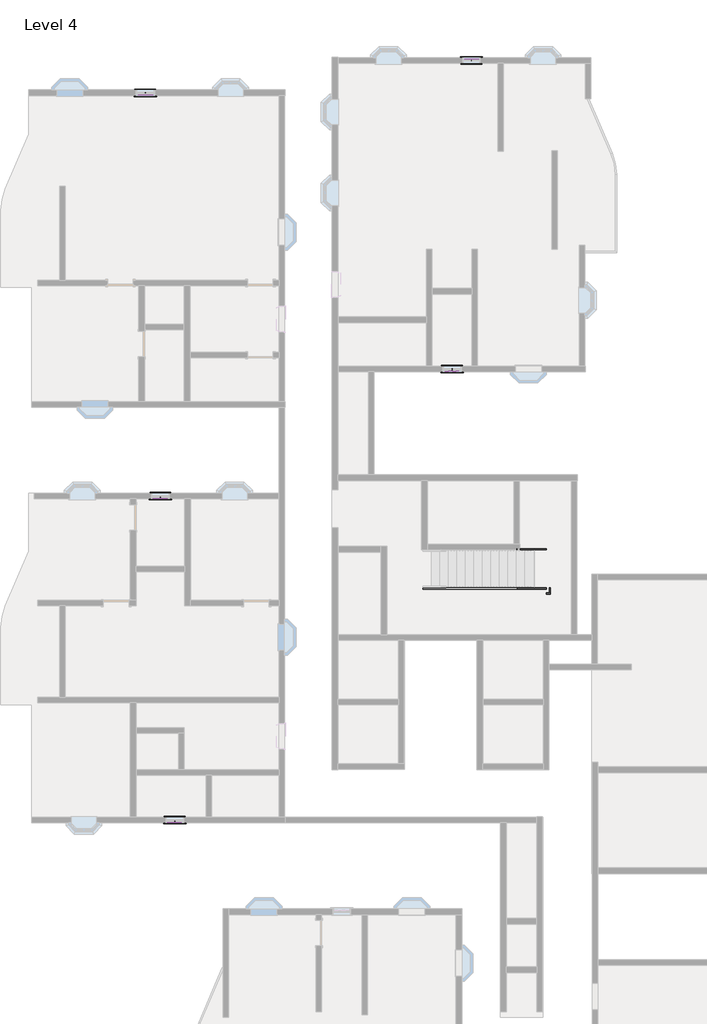
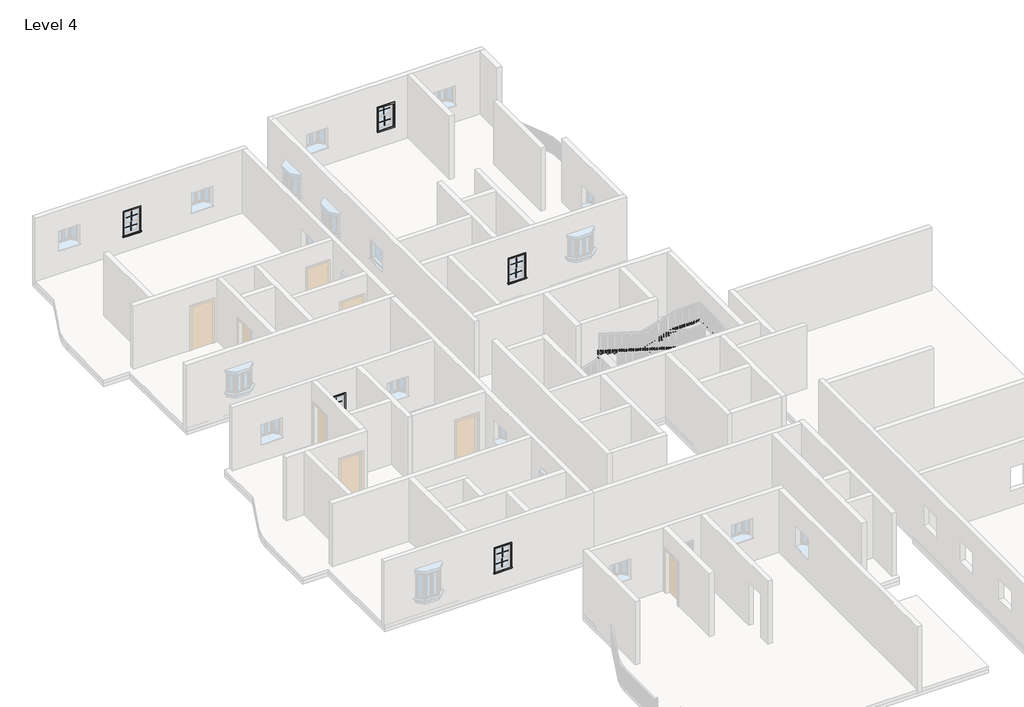
# One storey, part 14 of 14: 20 proxies, 6 members.
"""IFC4 building model written with IfcOpenShell, lengths in millimetres."""

from ifc_helpers import new_model, si_unit, frame, origin, place, context, project, spatial, polyline, outline, extrude, transform, mapped, element, save
from components import muntin_pattern_2x2_muntin_pattern_2x2_c35c595f, trim_window_exterior_flat_with_sill_e38017c9, trim_window_interior_flat_picture_frame_d728ed12

model = new_model("IFC4")

# Units and contexts
model_context = context("Model", 3, world=origin())
ifc_project = project(units=[si_unit("LENGTHUNIT", "METRE", prefix="MILLI")], contexts=[model_context])

# Site, building, storey
site = spatial("IfcSite", under=ifc_project)
building = spatial("IfcBuilding", under=site)
storey = spatial("IfcBuildingStorey", under=building, Name="Level 4", Elevation=9144.0)

# Proxies
placement = place(None, origin())
muntin_pattern_2x2_muntin_pattern_2x2_shape = muntin_pattern_2x2_muntin_pattern_2x2_c35c595f(model_context)
element("IfcBuildingElementProxy", 1, Name="Muntin Pattern_2x2 : Muntin Pattern_2x2", ObjectType="Muntin Pattern_2x2 : Muntin Pattern_2x2", at=placement, inside=storey, context=model_context, shape_type="MappedRepresentation", body=[
    mapped(muntin_pattern_2x2_muntin_pattern_2x2_shape, transform((-14639.3891351, 14368.0833494, 10614.025), x_axis=(-1.0, 0.0, 0.0), y_axis=(0.0, -1.0, 0.0), z_axis=(0.0, 0.0, 1.0))),
])
element("IfcBuildingElementProxy", 2, Name="Muntin Pattern_2x2 : Muntin Pattern_2x2", ObjectType="Muntin Pattern_2x2 : Muntin Pattern_2x2", at=placement, inside=storey, context=model_context, shape_type="MappedRepresentation", body=[
    mapped(muntin_pattern_2x2_muntin_pattern_2x2_shape, transform((-14639.3891351, 14412.5333494, 10134.6), x_axis=(-1.0, 0.0, 0.0), y_axis=(0.0, -1.0, 0.0), z_axis=(0.0, 0.0, 1.0))),
])
element("IfcBuildingElementProxy", 3, Name="Muntin Pattern_2x2 : Muntin Pattern_2x2", ObjectType="Muntin Pattern_2x2 : Muntin Pattern_2x2", at=placement, inside=storey, context=model_context, shape_type="MappedRepresentation", body=[
    mapped(muntin_pattern_2x2_muntin_pattern_2x2_shape, transform((-14125.0391351, 2785.6833494, 10614.025), x_axis=(-1.0, 0.0, 0.0), y_axis=(0.0, -1.0, 0.0), z_axis=(0.0, 0.0, 1.0))),
])
element("IfcBuildingElementProxy", 4, Name="Muntin Pattern_2x2 : Muntin Pattern_2x2", ObjectType="Muntin Pattern_2x2 : Muntin Pattern_2x2", at=placement, inside=storey, context=model_context, shape_type="MappedRepresentation", body=[
    mapped(muntin_pattern_2x2_muntin_pattern_2x2_shape, transform((-14125.0391351, 2830.1333494, 10134.6), x_axis=(-1.0, 0.0, 0.0), y_axis=(0.0, -1.0, 0.0), z_axis=(0.0, 0.0, 1.0))),
])
element("IfcBuildingElementProxy", 5, Name="Muntin Pattern_2x2 : Muntin Pattern_2x2", ObjectType="Muntin Pattern_2x2 : Muntin Pattern_2x2", at=placement, inside=storey, context=model_context, shape_type="MappedRepresentation", body=[
    mapped(muntin_pattern_2x2_muntin_pattern_2x2_shape, transform((-4206.3391351, 18910.0465905, 10614.025), x_axis=(-1.0, 0.0, 0.0), y_axis=(0.0, -1.0, 0.0), z_axis=(0.0, 0.0, 1.0))),
])
element("IfcBuildingElementProxy", 6, Name="Muntin Pattern_2x2 : Muntin Pattern_2x2", ObjectType="Muntin Pattern_2x2 : Muntin Pattern_2x2", at=placement, inside=storey, context=model_context, shape_type="MappedRepresentation", body=[
    mapped(muntin_pattern_2x2_muntin_pattern_2x2_shape, transform((-4206.3391351, 18954.4965905, 10134.6), x_axis=(-1.0, 0.0, 0.0), y_axis=(0.0, -1.0, 0.0), z_axis=(0.0, 0.0, 1.0))),
])
element("IfcBuildingElementProxy", 7, Name="Muntin Pattern_2x2 : Muntin Pattern_2x2", ObjectType="Muntin Pattern_2x2 : Muntin Pattern_2x2", at=placement, inside=storey, context=model_context, shape_type="MappedRepresentation", body=[
    mapped(muntin_pattern_2x2_muntin_pattern_2x2_shape, transform((-3514.1891351, 30066.9965905, 10614.025), x_axis=(1.0, 0.0, 0.0), y_axis=(0.0, 1.0, 0.0), z_axis=(0.0, 0.0, 1.0))),
])
element("IfcBuildingElementProxy", 8, Name="Muntin Pattern_2x2 : Muntin Pattern_2x2", ObjectType="Muntin Pattern_2x2 : Muntin Pattern_2x2", at=placement, inside=storey, context=model_context, shape_type="MappedRepresentation", body=[
    mapped(muntin_pattern_2x2_muntin_pattern_2x2_shape, transform((-3514.1891351, 30022.5465905, 10134.6), x_axis=(1.0, 0.0, 0.0), y_axis=(0.0, 1.0, 0.0), z_axis=(0.0, 0.0, 1.0))),
])
element("IfcBuildingElementProxy", 9, Name="Muntin Pattern_2x2 : Muntin Pattern_2x2", ObjectType="Muntin Pattern_2x2 : Muntin Pattern_2x2", at=placement, inside=storey, context=model_context, shape_type="MappedRepresentation", body=[
    mapped(muntin_pattern_2x2_muntin_pattern_2x2_shape, transform((-15175.9641351, 28782.5833494, 10614.025), x_axis=(-1.0, 0.0, 0.0), y_axis=(0.0, -1.0, 0.0), z_axis=(0.0, 0.0, 1.0))),
])
element("IfcBuildingElementProxy", 10, Name="Muntin Pattern_2x2 : Muntin Pattern_2x2", ObjectType="Muntin Pattern_2x2 : Muntin Pattern_2x2", at=placement, inside=storey, context=model_context, shape_type="MappedRepresentation", body=[
    mapped(muntin_pattern_2x2_muntin_pattern_2x2_shape, transform((-15175.9641351, 28827.0333494, 10134.6), x_axis=(-1.0, 0.0, 0.0), y_axis=(0.0, -1.0, 0.0), z_axis=(0.0, 0.0, 1.0))),
])
trim_window_exterior_flat_with_sill_shape = trim_window_exterior_flat_with_sill_e38017c9(model_context)
element("IfcBuildingElementProxy", 11, Name="Trim-Window-Exterior-Flat : with Sill", ObjectType="Trim-Window-Exterior-Flat : with Sill", at=placement, inside=storey, context=model_context, shape_type="MappedRepresentation", body=[
    mapped(trim_window_exterior_flat_with_sill_shape, transform((-14639.3891351, 14333.1583494, 11125.2), x_axis=(1.0, 0.0, 0.0), y_axis=(0.0, 0.0, 1.0), z_axis=(0.0, -1.0, 0.0))),
])
element("IfcBuildingElementProxy", 12, Name="Trim-Window-Exterior-Flat : with Sill", ObjectType="Trim-Window-Exterior-Flat : with Sill", at=placement, inside=storey, context=model_context, shape_type="MappedRepresentation", body=[
    mapped(trim_window_exterior_flat_with_sill_shape, transform((-14125.0391351, 2750.7583494, 11125.2), x_axis=(1.0, 0.0, 0.0), y_axis=(0.0, 0.0, 1.0), z_axis=(0.0, -1.0, 0.0))),
])
element("IfcBuildingElementProxy", 13, Name="Trim-Window-Exterior-Flat : with Sill", ObjectType="Trim-Window-Exterior-Flat : with Sill", at=placement, inside=storey, context=model_context, shape_type="MappedRepresentation", body=[
    mapped(trim_window_exterior_flat_with_sill_shape, transform((-4206.3391351, 18875.1215905, 11125.2), x_axis=(1.0, 0.0, 0.0), y_axis=(0.0, 0.0, 1.0), z_axis=(0.0, -1.0, 0.0))),
])
element("IfcBuildingElementProxy", 14, Name="Trim-Window-Exterior-Flat : with Sill", ObjectType="Trim-Window-Exterior-Flat : with Sill", at=placement, inside=storey, context=model_context, shape_type="MappedRepresentation", body=[
    mapped(trim_window_exterior_flat_with_sill_shape, transform((-3514.1891351, 30101.9215905, 11125.2), x_axis=(-1.0, 0.0, 0.0), y_axis=(0.0, 0.0, 1.0), z_axis=(0.0, 1.0, 0.0))),
])
element("IfcBuildingElementProxy", 15, Name="Trim-Window-Exterior-Flat : with Sill", ObjectType="Trim-Window-Exterior-Flat : with Sill", at=placement, inside=storey, context=model_context, shape_type="MappedRepresentation", body=[
    mapped(trim_window_exterior_flat_with_sill_shape, transform((-15175.9641351, 28747.6583494, 11125.2), x_axis=(1.0, 0.0, 0.0), y_axis=(0.0, 0.0, 1.0), z_axis=(0.0, -1.0, 0.0))),
])
trim_window_interior_flat_picture_frame_shape = trim_window_interior_flat_picture_frame_d728ed12(model_context)
element("IfcBuildingElementProxy", 16, Name="Trim-Window-Interior-Flat : Picture Frame", ObjectType="Trim-Window-Interior-Flat : Picture Frame", at=placement, inside=storey, context=model_context, shape_type="MappedRepresentation", body=[
    mapped(trim_window_interior_flat_picture_frame_shape, transform((-14639.3891351, 14536.3583494, 11125.2), x_axis=(-1.0, 0.0, 0.0), y_axis=(0.0, 0.0, 1.0), z_axis=(0.0, 1.0, 0.0))),
])
element("IfcBuildingElementProxy", 17, Name="Trim-Window-Interior-Flat : Picture Frame", ObjectType="Trim-Window-Interior-Flat : Picture Frame", at=placement, inside=storey, context=model_context, shape_type="MappedRepresentation", body=[
    mapped(trim_window_interior_flat_picture_frame_shape, transform((-14125.0391351, 2953.9583494, 11125.2), x_axis=(-1.0, 0.0, 0.0), y_axis=(0.0, 0.0, 1.0), z_axis=(0.0, 1.0, 0.0))),
])
element("IfcBuildingElementProxy", 18, Name="Trim-Window-Interior-Flat : Picture Frame", ObjectType="Trim-Window-Interior-Flat : Picture Frame", at=placement, inside=storey, context=model_context, shape_type="MappedRepresentation", body=[
    mapped(trim_window_interior_flat_picture_frame_shape, transform((-4206.3391351, 19078.3215905, 11125.2), x_axis=(-1.0, 0.0, 0.0), y_axis=(0.0, 0.0, 1.0), z_axis=(0.0, 1.0, 0.0))),
])
element("IfcBuildingElementProxy", 19, Name="Trim-Window-Interior-Flat : Picture Frame", ObjectType="Trim-Window-Interior-Flat : Picture Frame", at=placement, inside=storey, context=model_context, shape_type="MappedRepresentation", body=[
    mapped(trim_window_interior_flat_picture_frame_shape, transform((-3514.1891351, 29898.7215905, 11125.2), x_axis=(1.0, 0.0, 0.0), y_axis=(0.0, 0.0, 1.0), z_axis=(0.0, -1.0, 0.0))),
])
element("IfcBuildingElementProxy", 20, Name="Trim-Window-Interior-Flat : Picture Frame", ObjectType="Trim-Window-Interior-Flat : Picture Frame", at=placement, inside=storey, context=model_context, shape_type="MappedRepresentation", body=[
    mapped(trim_window_interior_flat_picture_frame_shape, transform((-15175.9641351, 28950.8583494, 11125.2), x_axis=(-1.0, 0.0, 0.0), y_axis=(0.0, 0.0, 1.0), z_axis=(0.0, 1.0, 0.0))),
])

# Members
element("IfcMember", 21, ObjectType="Stringer - 2\" Width", at=placement, inside=storey, context=model_context, shape_type="SweptSolid", body=[
    extrude(outline(polyline([(9335.5995961, -5254.0891351), (9144.0, -5254.0891351), (9144.0, -4832.019314), (10591.8, -6.019314), (10591.8, -1066.7544553), (9335.5995961, -5254.0891351)])), frame((0.0, 12506.0715905, 0.0), z_axis=(0.0, 1.0, 0.0), x_axis=(0.0, 0.0, 1.0)), (0.0, 0.0, 1.0), 50.8),
])
element("IfcMember", 22, ObjectType="Stringer - 2\" Width", at=placement, inside=storey, context=model_context, shape_type="SweptSolid", body=[
    extrude(outline(polyline([(54.5108649, 12556.8715905), (105.3108649, 12556.8715905), (105.3108649, 9478.4949943), (54.5108649, 9478.4949943), (54.5108649, 12556.8715905)])), frame((0.0, 0.0, 10287.0), z_axis=(0.0, 0.0, 1.0), x_axis=(1.0, 0.0, 0.0)), (0.0, 0.0, 1.0), 304.8),
])
element("IfcMember", 23, ObjectType="Stringer - 2\" Width", at=placement, inside=storey, context=model_context, shape_type="SweptSolid", body=[
    extrude(outline(polyline([(10287.0, 105.3108649), (10379.5395961, 105.3108649), (11987.3595961, -5254.0891351), (11669.1390537, -5254.0891351), (10287.0, -646.9589562), (10287.0, 105.3108649)])), frame((0.0, 9427.6949943, 0.0), z_axis=(0.0, 1.0, 0.0), x_axis=(0.0, 0.0, 1.0)), (0.0, 0.0, 1.0), 50.8),
])
element("IfcMember", 24, ObjectType="Stringer - 2\" Width", at=placement, inside=storey, context=model_context, shape_type="SweptSolid", body=[
    extrude(outline(polyline([(9335.5995961, -5254.0891351), (9144.0, -5254.0891351), (9144.0, -4832.019314), (10373.7390537, -732.8891351), (10591.8, -732.8891351), (10591.8, -1066.7544553), (9335.5995961, -5254.0891351)])), frame((0.0, 11103.4082924, 0.0), z_axis=(0.0, 1.0, 0.0), x_axis=(0.0, 0.0, 1.0)), (0.0, 0.0, 1.0), 50.8),
])
element("IfcMember", 25, ObjectType="Stringer - 2\" Width", at=placement, inside=storey, context=model_context, shape_type="SweptSolid", body=[
    extrude(outline(polyline([(-732.8891351, 11154.2082924), (-682.0891351, 11154.2082924), (-682.0891351, 10976.4082924), (-732.8891351, 10976.4082924), (-732.8891351, 11154.2082924)])), frame((0.0, 0.0, 10287.0), z_axis=(0.0, 0.0, 1.0), x_axis=(1.0, 0.0, 0.0)), (0.0, 0.0, 1.0), 304.8),
])
element("IfcMember", 26, ObjectType="Stringer - 2\" Width", at=placement, inside=storey, context=model_context, shape_type="SweptSolid", body=[
    extrude(outline(polyline([(10297.5390537, -682.0891351), (10615.7595961, -682.0891351), (11987.3595961, -5254.0891351), (11669.1390537, -5254.0891351), (10297.5390537, -682.0891351)])), frame((0.0, 10925.6082924, 0.0), z_axis=(0.0, 1.0, 0.0), x_axis=(0.0, 0.0, 1.0)), (0.0, 0.0, 1.0), 50.8),
])

save(model, "model.ifc")

# Revit data of these elements
# Type "Muntin Pattern_2x2 : Muntin Pattern_2x2"
#   Width [instance default] = 4' - 0"
#   Thickness = 0' - 0 1/2"
#   Height [instance default] = 4' - 0"
#   Distance = 0' - 0 3/4"
#   Interior Material [instance default] = none
#   Exterior Material [instance default] = none
#   Default Elevation = 0
# Type "Trim-Window-Exterior-Flat : with Sill"
#   Trim Width = 0' - 2 1/4"
#   Trim Thickness_Picture Frame = 0' - 1 1/4"
#   Trim Thickness_with Sill = 0' - 0 3/4"
#   Sill Thickness = 0' - 1 1/4"
#   Opening Width [instance default] = 2' - 0"
#   Opening Height [instance default] = 3' - 0"
#   Default Elevation = 4' - 0"
#   Sill = yes
#   Picture Frame = no
#   Trim Material [instance default] = none
# Type "Trim-Window-Interior-Flat : Picture Frame"
#   Trim Thickness_Picture Frame = 0' - 1 1/4"
#   Trim Width = 0' - 2 1/4"
#   Trim Thickness_with Sill = 0' - 0 3/4"
#   Sill Thickness = 0' - 1 1/4"
#   Opening Width [instance default] = 2' - 0"
#   Opening Height [instance default] = 3' - 0"
#   Default Elevation = 4' - 0"
#   Sill = no
#   Picture Frame = yes
#   Trim Material [instance default] = none
# Elements 1, 2, 3, 4, 5, 6, 7, 8, 9, 10 (IfcBuildingElementProxy, "Muntin Pattern_2x2 : Muntin Pattern_2x2")
#   Width = 1' - 8"
#   Height = 1' - 5 1/8"
#   Interior Material = Wood - Stained
#   Exterior Material = Clad - White
#   Phase Created = New Construction
#   Materials on its faces: "Clad - White", "Wood - Stained"
# Elements 11, 12, 13, 14, 15 (IfcBuildingElementProxy, "Trim-Window-Exterior-Flat : with Sill")
#   Opening Width = 2' - 2"
#   Opening Height = 3' - 6"
#   Trim Material = Clad - White
#   Phase Created = New Construction
#   Materials on its faces: "Clad - White"
# Elements 16, 17, 18, 19, 20 (IfcBuildingElementProxy, "Trim-Window-Interior-Flat : Picture Frame")
#   Opening Width = 2' - 2"
#   Opening Height = 3' - 6"
#   Trim Material = Wood - Stained
#   Phase Created = New Construction
#   Materials on its faces: "Wood - Stained"
# Elements 21, 22, 23, 24, 25, 26 (IfcMember, "Stringer - 2\" Width")
#   Phase Created = New Construction
# Materials
#   "Clad - White": class "Wood", colour RGB 242 242 238, transparency 0, Cost = 0
#   "Wood - Stained": class "Wood", colour RGB 224 178 126, transparency 0, Cost = 0
